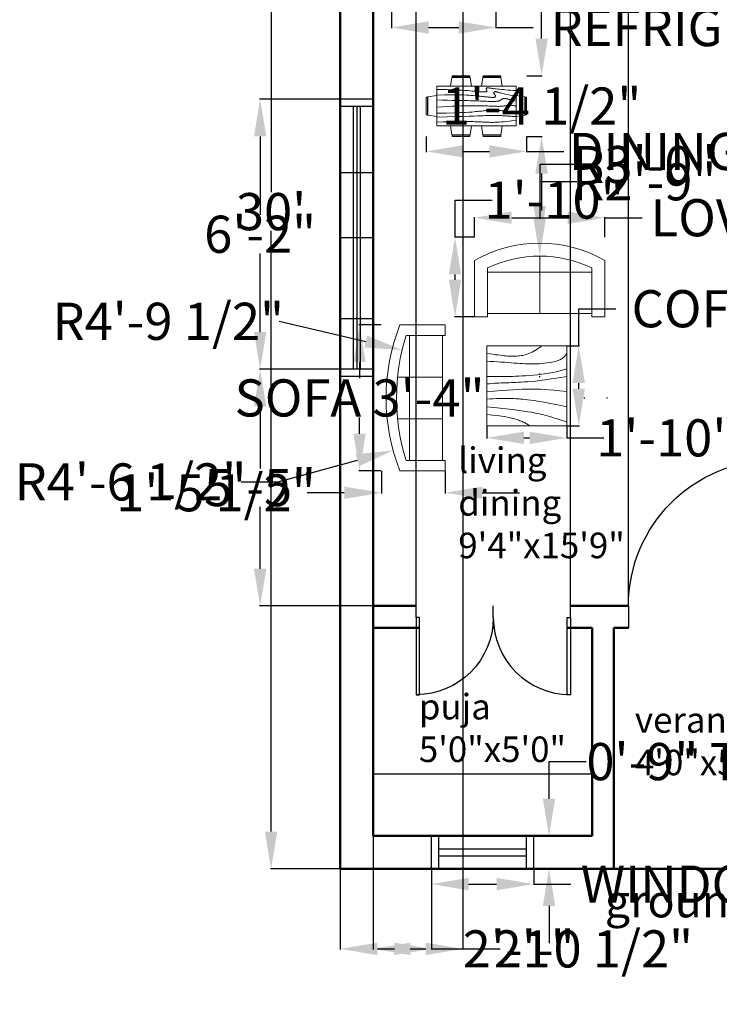
# Model space of a CAD drawing. Units: inches. Extents: x 19 to 1371, y 7 to 588.
# Tile 1 of 5: x 879 to 1070, y 103 to 372. Entities that reach past the tile are written whole.
import ezdxf

# ---------------------------------------------------------------- set-up
doc = ezdxf.new("R2010")
doc.units = ezdxf.units.IN
doc.header["$MEASUREMENT"] = 0
for name, color, linetype, lineweight in [('A-ANNO-DIMS', 2, 'Continuous', 18), ('A-ANNO-TEXT', 7, 'Continuous', 18), ('A-AREA-IDEN', 7, 'Continuous', 18), ('A-DOOR', 3, 'Continuous', 25), ('A-FLOR-CABN', 8, 'Continuous', 25), ('A-FURN', 8, 'Continuous', 18), ('A-GLAZ', 4, 'Continuous', 25), ('A-WALL', 7, 'Continuous', 50)]:
    doc.layers.add(name, color=color, linetype=linetype, lineweight=lineweight)
doc.styles.get("Standard").update_dxf_attribs({"font": 'arial.ttf'})
doc.dimstyles.get("Standard").update_dxf_attribs({"dimtxt": 10.18, "dimasz": 10.18, "dimexe": 0.18, "dimexo": 0.0625, "dimgap": 0.09, "dimtad": 0, "dimtih": 1, "dimtoh": 1, "dimdec": 0, "dimzin": 0, "dimdsep": 46, "dimlunit": 3, "dimtxsty": 'Standard', "dimcen": 0.09, "dimadec": 0, "dimazin": 0, "dimtfac": 1, "dimtdec": 0, "dimtofl": 0, "dimtmove": 0, "dimatfit": 3, "dimfxl": 1, "dimtolj": 1, "dimtzin": 0, "dimarcsym": 0})

# ---------------------------------------------------------------- blocks, each defined once
blk = doc.blocks.new('*U2')
for p, q in [((0, 0), (0, -6)), ((40, 0), (40, -6))]:
    blk.add_line(p, q)
blk.add_lwpolyline([(0, 0), (0, 40), (1.75, 40), (1.75, 0)], close=True)
blk.add_arc((0, 0), 40, 0, 90)
blk = doc.blocks.new('Dining Set - 36 x 72 in.')
for p, q in [((-22, 27.5), (-22.1562, 26.50042)), ((-22, 27.5), (-6, 27.5)), ((-5.8437, 26.49966), (-6, 27.5)), ((6, 27.5), (5.8438, 26.50042)), ((6, 27.5), (22, 27.5)), ((22.1563, 26.49966), (22, 27.5)), ((36, 18), (-36, 18)), ((-36, 18), (-36, -18)), ((-22.2343, 26.00059), (-23.4847, 17.99762)), ((-22.2304, 26), (-5.7608, 26)), ((-5.8416, 26.5), (-22.1534, 26.5)), ((-4.5152, 17.99762), (-5.7655, 25.99926)), ((5.7657, 26.00059), (4.5153, 17.99762)), ((5.7696, 26), (22.2392, 26)), ((22.1584, 26.5), (5.8466, 26.5)), ((23.4848, 17.99762), (22.2345, 25.99926)), ((36, -18), (36, 18)), ((-44.0006, 8.23428), (-35.9976, 9.48474)), ((44.0006, 8.23428), (35.9976, 9.48474)), ((-45.5, 8), (-44.5004, 8.15617)), ((-45.5, 8), (-45.5, -8)), ((-44.5, -8.15843), (-44.5, 8.15338)), ((-44, 8.23041), (-44, -8.23915)), ((44, 8.23041), (44, -8.23915)), ((44.5, -8.15843), (44.5, 8.15338)), ((45.5, 8), (44.5005, 8.15617)), ((45.5, 8), (45.5, -8)), ((-44.4997, -8.15631), (-45.5, -8)), ((-35.9976, -9.48476), (-43.9993, -8.2345)), ((35.9976, -9.48476), (43.9993, -8.2345)), ((44.4997, -8.15631), (45.5, -8)), ((-36, -18), (36, -18)), ((-22.2343, -26.0006), (-23.4847, -17.99762)), ((-22.2304, -26), (-5.7608, -26)), ((-22, -27.5), (-22.1562, -26.50044)), ((-5.8416, -26.5), (-22.1534, -26.5)), ((-5.8437, -26.49967), (-6, -27.5)), ((-4.5152, -17.99762), (-5.7655, -25.99928)), ((5.7657, -26.0006), (4.5153, -17.99762)), ((5.7696, -26), (22.2392, -26)), ((6, -27.5), (5.8438, -26.50044)), ((22.1584, -26.5), (5.8466, -26.5)), ((22.1563, -26.49967), (22, -27.5)), ((23.4848, -17.99762), (22.2345, -25.99928)), ((-22, -27.5), (-6, -27.5)), ((6, -27.5), (22, -27.5))]:
    blk.add_line(p, q)
for points in [[(-36, 15), (-31.1772, 14.97754), (-26.8079, 14.91406), (-22.8538, 14.81543), (-19.276, 14.6875), (-16.0362, 14.53613), (-13.0957, 14.36718), (-10.4159, 14.18652), (-7.9583, 14), (-5.6904, 13.81315), (-3.6035, 13.63021), (-1.6954, 13.45508), (0.0365, 13.29166), (1.5945, 13.14388), (2.9811, 13.01562), (4.1988, 12.9108), (5.25, 12.83333), (6.1393, 12.78613), (6.8802, 12.76823), (7.4883, 12.77767), (7.9792, 12.8125), (8.3685, 12.87077), (8.6719, 12.95052), (8.9049, 13.0498), (9.0833, 13.16666), (9.2205, 13.29899), (9.3216, 13.44401), (9.3895, 13.59879), (9.4271, 13.76041), (9.4373, 13.92594), (9.4232, 14.09245), (9.3875, 14.257), (9.3333, 14.41666), (9.2638, 14.56917), (9.1836, 14.71484), (9.0975, 14.85465), (9.0104, 14.98958), (8.9272, 15.1206), (8.8529, 15.2487), (8.7922, 15.37483), (8.75, 15.5), (8.7305, 15.62467), (8.7344, 15.74739), (8.7617, 15.86621), (8.8125, 15.97916), (8.8867, 16.08431), (8.9844, 16.17968), (9.1055, 16.26334), (9.25, 16.33333), (9.4189, 16.38802), (9.6172, 16.42708), (9.8506, 16.45052), (10.125, 16.45833), (10.4463, 16.45052), (10.8203, 16.42708), (11.2529, 16.38802), (11.75, 16.33333), (12.3184, 16.26318), (12.9694, 16.17838), (13.7151, 16.07991), (14.5677, 15.96875), (15.5395, 15.84586), (16.6426, 15.71224), (17.8893, 15.56884), (19.2917, 15.41666), (20.859, 15.25667), (22.5879, 15.08984), (24.4721, 14.91715), (26.5052, 14.73958), (28.6809, 14.5581), (30.9929, 14.3737), (33.4347, 14.18733), (36, 14)], [(-36, 10), (-28.9766, 10.14274), (-23.1725, 10.20442), (-18.4241, 10.19775), (-14.5677, 10.13541), (-11.4399, 10.03011), (-8.877, 9.89453), (-6.7154, 9.74137), (-4.7917, 9.58333), (-2.9698, 9.43082), (-1.2246, 9.28515), (0.4415, 9.14534), (2.026, 9.01041), (3.5266, 8.87939), (4.9408, 8.7513), (6.266, 8.62516), (7.5, 8.5), (8.6411, 8.37549), (9.6914, 8.2539), (10.6538, 8.13818), (11.5312, 8.03125), (12.3267, 7.93603), (13.043, 7.85547), (13.6831, 7.79248), (14.25, 7.75), (14.7471, 7.7303), (15.1797, 7.73307), (15.5537, 7.75732), (15.875, 7.80208), (16.1494, 7.86637), (16.3828, 7.94922), (16.5811, 8.04964), (16.75, 8.16666), (16.8944, 8.29915), (17.0143, 8.44531), (17.1089, 8.60319), (17.1771, 8.77083), (17.218, 8.94629), (17.2305, 9.1276), (17.2137, 9.31282), (17.1667, 9.5), (17.0895, 9.6875), (16.987, 9.875), (16.8649, 10.0625), (16.7292, 10.25), (16.5856, 10.4375), (16.4401, 10.625), (16.2985, 10.8125), (16.1667, 11), (16.05, 11.18733), (15.9518, 11.3737), (15.8752, 11.5581), (15.8229, 11.73958), (15.798, 11.91715), (15.8034, 12.08984), (15.842, 12.25667), (15.9167, 12.41666), (16.0295, 12.56836), (16.1784, 12.70833), (16.3605, 12.83268), (16.5729, 12.9375), (16.8127, 13.01888), (17.0768, 13.07291), (17.3625, 13.0957), (17.6667, 13.08333), (17.9894, 13.03312), (18.3418, 12.94726), (18.7382, 12.82918), (19.1927, 12.68229), (19.7195, 12.51001), (20.3327, 12.31575), (21.0465, 12.10294), (21.875, 11.875), (22.8357, 11.63354), (23.959, 11.37304), (25.2786, 11.08618), (26.8282, 10.76562), (28.6414, 10.40405), (30.752, 9.99414), (33.1936, 9.52856), (36, 9)], [(-36, 5.5), (-30.7157, 5.3348), (-26.069, 5.20963), (-21.9946, 5.11767), (-18.4271, 5.05208), (-15.3009, 5.00602), (-12.5508, 4.97265), (-10.1112, 4.94515), (-7.9167, 4.91666), (-5.909, 4.88167), (-4.0586, 4.83984), (-2.3429, 4.79215), (-0.7396, 4.73958), (0.7739, 4.6831), (2.22, 4.6237), (3.6213, 4.56233), (5, 4.5), (6.373, 4.43782), (7.7344, 4.3776), (9.0723, 4.32129), (10.375, 4.27083), (11.6309, 4.22819), (12.8281, 4.19531), (13.9551, 4.17415), (15, 4.16666), (15.954, 4.17448), (16.819, 4.19791), (17.6001, 4.23698), (18.3021, 4.29166), (18.9299, 4.36198), (19.4883, 4.44791), (19.9823, 4.54948), (20.4167, 4.66666), (20.7969, 4.79899), (21.1302, 4.94401), (21.4245, 5.09879), (21.6875, 5.26041), (21.9271, 5.42594), (22.1511, 5.59245), (22.3672, 5.757), (22.5834, 5.91666), (22.8065, 6.06868), (23.0404, 6.21093), (23.2879, 6.34147), (23.5521, 6.45833), (23.8358, 6.55957), (24.142, 6.64323), (24.4735, 6.70735), (24.8334, 6.75), (25.2235, 6.76969), (25.642, 6.76692), (26.0858, 6.74267), (26.5521, 6.69791), (27.0379, 6.63362), (27.5404, 6.55078), (28.0565, 6.45036), (28.5834, 6.33333), (29.1242, 6.19987), (29.7071, 6.04687), (30.3661, 5.87044), (31.1354, 5.66666), (32.0493, 5.43164), (33.142, 5.16146), (34.4475, 4.85221), (36, 4.5)], [(-36, -1), (-30.7915, -0.6591), (-26.0195, -0.38216), (-21.6519, -0.16284), (-17.6563, 0.00521), (-14.0005, 0.12833), (-10.6523, 0.21289), (-7.5796, 0.26522), (-4.75, 0.29166), (-2.134, 0.29793), (0.2878, 0.28711), (2.5317, 0.26163), (4.6146, 0.22396), (6.5529, 0.17651), (8.3633, 0.12174), (10.0623, 0.06209), (11.6667, 0), (13.1899, -0.06201), (14.6341, -0.1211), (15.9982, -0.17432), (17.2813, -0.21875), (18.4823, -0.25147), (19.6003, -0.26953), (20.6343, -0.27002), (21.5834, -0.25), (22.4481, -0.20768), (23.2357, -0.14584), (23.9549, -0.06836), (24.6146, 0.02083), (25.2235, 0.11784), (25.7904, 0.21875), (26.3241, 0.31966), (26.8334, 0.41666), (27.3265, 0.50618), (27.8099, 0.58593), (28.2894, 0.65397), (28.7709, 0.70833), (29.2601, 0.74707), (29.763, 0.76823), (30.2855, 0.76985), (30.8334, 0.75), (31.4088, 0.70784), (31.9994, 0.64713), (32.589, 0.57275), (33.1615, 0.48958), (33.7008, 0.4025), (34.1908, 0.3164), (34.6153, 0.23616), (34.9584, 0.16666), (35.2099, 0.11165), (35.3848, 0.07031), (35.504, 0.04069), (35.5886, 0.02083), (35.6594, 0.00879), (35.7377, 0.0026), (35.8442, 0.00032), (36, 0)], [(-36, -6.5), (-27.1843, -6.31267), (-20.084, -6.1263), (-14.469, -5.9419), (-10.1094, -5.76042), (-6.7752, -5.58285), (-4.2363, -5.41016), (-2.2629, -5.24333), (-0.625, -5.08334), (0.8708, -4.93099), (2.2715, -4.78646), (3.5872, -4.64974), (4.8281, -4.52084), (6.0046, -4.39974), (7.127, -4.28646), (8.2053, -4.18099), (9.25, -4.08334), (10.2705, -3.99382), (11.2734, -3.91407), (12.2647, -3.84603), (13.25, -3.79167), (14.2354, -3.75293), (15.2266, -3.73177), (16.2295, -3.73015), (17.25, -3.75), (18.2912, -3.79248), (19.3451, -3.85547), (20.4009, -3.93604), (21.4479, -4.03125), (22.4754, -4.13819), (23.4727, -4.25391), (24.4289, -4.37549), (25.3334, -4.5), (26.1785, -4.62492), (26.9694, -4.74935), (27.7145, -4.87281), (28.4219, -4.99479), (29.1, -5.11483), (29.7572, -5.23242), (30.4016, -5.34709), (31.0417, -5.45834), (31.6837, -5.56437), (32.3262, -5.65821), (32.9658, -5.73153), (33.599, -5.77604), (34.2224, -5.78345), (34.8327, -5.74545), (35.4264, -5.65373), (36, -5.5)], [(-36, -10), (-26.4022, -9.81299), (-18.4675, -9.62891), (-11.9839, -9.45069), (-6.7396, -9.28125), (-2.5226, -9.12354), (0.8789, -8.98047), (3.6769, -8.85498), (6.0833, -8.75), (8.2767, -8.66765), (10.3021, -8.60677), (12.1712, -8.56543), (13.8958, -8.54167), (15.4876, -8.53353), (16.9583, -8.53907), (18.3197, -8.55632), (19.5834, -8.58334), (20.7616, -8.61841), (21.8685, -8.66081), (22.9188, -8.71004), (23.9271, -8.76563), (24.9081, -8.82707), (25.8763, -8.89388), (26.8465, -8.96558), (27.8334, -9.04167), (28.8474, -9.12118), (29.8828, -9.20117), (30.93, -9.27824), (31.9792, -9.34896), (33.0205, -9.40991), (34.0443, -9.45768), (35.0407, -9.48885), (36, -9.5)], [(-36, -14.5), (-30.0881, -14.33513), (-25.0332, -14.21224), (-20.7312, -14.12647), (-17.0781, -14.07292), (-13.97, -14.04671), (-11.3027, -14.04297), (-8.9724, -14.05681), (-6.875, -14.08334), (-4.9224, -14.11833), (-3.0905, -14.16016), (-1.3709, -14.20785), (0.2448, -14.26042), (1.7647, -14.3169), (3.1973, -14.3763), (4.5507, -14.43767), (5.8333, -14.5), (7.0554, -14.5621), (8.235, -14.62175), (9.3922, -14.67652), (10.5469, -14.72396), (11.7192, -14.76164), (12.929, -14.78711), (14.1965, -14.79794), (15.5417, -14.79167), (16.9933, -14.76424), (18.6152, -14.70508), (20.4804, -14.60197), (22.6615, -14.44271), (25.2312, -14.21509), (28.2624, -13.9069), (31.8277, -13.50594), (36, -13)]]:
    blk.add_lwpolyline(points)
blk = doc.blocks.new('Sofa - Roundback 7 ft.')
for p, q in [((-12.00002, -32.4421), (-12.00003, -6.5971)), ((11.99997, -32.4421), (11.99998, -6.5971)), ((-36.000027, -34), (-36.000027, -11.4696)), ((-35.999844, -13.3819), (35.9998, -13.3819)), ((35.99998, -34), (35.99998, -11.4696)), ((-36.000027, -32.4421), (35.99998, -32.4421))]:
    blk.add_line(p, q)
for points in [[(-36.000027, -34), (-42.000027, -34), (-42.000027, -8)], [(41.99998, -8), (41.99998, -34), (35.99998, -34)]]:
    blk.add_lwpolyline(points)
for centre, radius, start, end in [((0, -114.25), 114.25, 68.43141, 111.5686), ((-0.00001, -127.1968), 121.1968, 72.72033, 107.2797)]:
    blk.add_arc(centre, radius, start, end)
blk = doc.blocks.new('Sofa - Roundback Loveseat 5 ft.')
for p, q in [((0, -32.44198), (0, -5.99998)), ((-24, -33.99998), (-24, -11.46958)), ((-23.9998, -13.38178), (23.99986, -13.38178)), ((24.00004, -33.99998), (24.00004, -11.46958)), ((-24, -32.44198), (24.00004, -32.44198))]:
    blk.add_line(p, q)
for points in [[(-24, -33.99998), (-30, -33.99998), (-30, -7.99998)], [(30.00004, -7.99998), (30.00004, -33.99998), (24.00004, -33.99998)]]:
    blk.add_lwpolyline(points)
for centre, radius, start, end in [((0, -60.24998), 60.24998, 60.13715, 119.8628), ((0, -61.38438), 55.38444, 64.32083, 115.6792)]:
    blk.add_arc(centre, radius, start, end)
blk = doc.blocks.new('Table - Square Woodgrain 42 x 42 in.')
blk.add_line((0, -42), (42, -42))
for points in [[(0, -4), (1.704, -4.2172), (3.2358, -4.4188), (4.615, -4.604), (5.8615, -4.7721), (6.9951, -4.9224), (8.0357, -5.0541), (9.0031, -5.1667), (9.9171, -5.2594), (10.7951, -5.3316), (11.6445, -5.3836), (12.4702, -5.4157), (13.277, -5.4283), (14.0698, -5.4217), (14.8535, -5.3964), (15.6331, -5.3526), (16.4133, -5.2908), (17.1986, -5.2103), (17.9913, -5.1062), (18.793, -4.9727), (19.6056, -4.8038), (20.4307, -4.5937), (21.2701, -4.3365), (22.1256, -4.0262), (22.9989, -3.6571), (23.888, -3.2272), (24.7756, -2.7516), (25.6408, -2.2491), (26.4624, -1.7387), (27.2195, -1.2395), (27.891, -0.7703), (28.456, -0.3501), (28.8934, 0.002)], [(0, -42), (0, 0), (42, 0), (42, -42)], [(0, -8), (1.8203, -8.1001), (3.6741, -8.2149), (5.5411, -8.3408), (7.4011, -8.4741), (9.2339, -8.6112), (11.0193, -8.7484), (12.7371, -8.8821), (14.3671, -9.0086), (15.8954, -9.1246), (17.3337, -9.2278), (18.6997, -9.3159), (20.0116, -9.387), (21.2871, -9.4389), (22.5442, -9.4696), (23.8008, -9.477), (25.0749, -9.459), (26.3791, -9.4137), (27.7049, -9.3403), (29.0383, -9.2382), (30.3655, -9.1068), (31.6728, -8.9455), (32.9461, -8.7535), (34.1717, -8.5304), (35.3358, -8.2756), (36.4268, -7.9863), (37.443, -7.6521), (38.3849, -7.2603), (39.253, -6.7986), (40.048, -6.2542), (40.7705, -5.6147), (41.421, -4.8674), (42, -4)], [(42, -12), (39.1784, -12.8621), (36.4519, -13.5654), (33.8246, -14.1294), (31.3004, -14.5731), (28.8832, -14.9161), (26.577, -15.1775), (24.3858, -15.3768), (22.3136, -15.5332), (20.3622, -15.6632), (18.5254, -15.7718), (16.7947, -15.8612), (15.1618, -15.9338), (13.6183, -15.9916), (12.1558, -16.0369), (10.7659, -16.0718), (9.4403, -16.0987), (8.1703, -16.1191), (6.9461, -16.1325), (5.7577, -16.1377), (4.595, -16.1335), (3.4479, -16.1188), (2.3064, -16.0924), (1.1604, -16.0532), (0, -16)], [(42, -16), (37.6529, -16.7365), (33.8802, -17.329), (30.6179, -17.7961), (27.8015, -18.1561), (25.3668, -18.4275), (23.2497, -18.6288), (21.3859, -18.7785), (19.7111, -18.8949), (18.1693, -18.9939), (16.7375, -19.0795), (15.401, -19.1534), (14.1449, -19.217), (12.9544, -19.2717), (11.8148, -19.3191), (10.7113, -19.3606), (9.6291, -19.3976), (8.5534, -19.4323), (7.47, -19.4689), (6.3643, -19.5122), (5.222, -19.5672), (4.0288, -19.6386), (2.7703, -19.7313), (1.4321, -19.8501), (0, -20)], [(0, -24), (3.9243, -23.6805), (7.4766, -23.4138), (10.6891, -23.1954), (13.5943, -23.0205), (16.2247, -22.8847), (18.6125, -22.7832), (20.7903, -22.7116), (22.7903, -22.6651), (24.6563, -22.642), (26.4764, -22.6507), (28.35, -22.7024), (30.3766, -22.8084), (32.6555, -22.98), (35.2861, -23.2283), (38.3678, -23.5645), (42, -24)], [(42, -32), (37.392, -31.017), (33.4585, -30.2231), (30.1291, -29.5949), (27.3334, -29.109), (25.0009, -28.742), (23.0612, -28.4707), (21.4439, -28.2716), (20.0786, -28.1215), (18.8998, -28.0002), (17.8609, -27.9014), (16.9206, -27.8219), (16.0371, -27.7588), (15.1691, -27.709), (14.2748, -27.6693), (13.3128, -27.6368), (12.2415, -27.6083), (11.0295, -27.5824), (9.6867, -27.5643), (8.233, -27.5608), (6.6884, -27.5787), (5.0728, -27.6248), (3.4062, -27.7058), (1.7086, -27.8286), (0, -28)], [(0, -32), (5.4026, -32.5358), (9.9494, -33.019), (13.7424, -33.4553), (16.8834, -33.8505), (19.4743, -34.2106), (21.6171, -34.5413), (23.4136, -34.8486), (24.9657, -35.1382), (26.3614, -35.4156), (27.6332, -35.6841), (28.7995, -35.9467), (29.8788, -36.2064), (30.8897, -36.4661), (31.8507, -36.7288), (32.7802, -36.9973), (33.6968, -37.2747), (34.6175, -37.5635), (35.5531, -37.8651), (36.5128, -38.1805), (37.506, -38.5108), (38.5421, -38.8568), (39.6302, -39.2197), (40.7797, -39.6004), (42, -40)], [(0, -36), (3.0098, -36.2857), (5.5354, -36.5643), (7.6368, -36.8359), (9.374, -37.1009), (10.807, -37.3597), (11.9957, -37.6126), (13.0002, -37.8599), (13.8804, -38.102), (14.6874, -38.3393), (15.4365, -38.5729), (16.1338, -38.8041), (16.7858, -39.0341), (17.3987, -39.264), (17.9787, -39.4952), (18.5322, -39.7288), (19.0655, -39.9662), (19.5832, -40.2081), (20.0842, -40.4544), (20.5657, -40.7046), (21.0249, -40.9581), (21.459, -41.2144), (21.8653, -41.4731), (22.2409, -41.7335), (22.5831, -41.9951)]]:
    blk.add_lwpolyline(points)
blk = doc.blocks.new('*D14')
at = {"layer": 'A-ANNO-DIMS', "color": 0, "lineweight": -2, "transparency": 16777216}
for p, q in [((966.38, 499.95), (947.31, 499.95)), ((947.49, 489.77), (947.49, 325.21)), ((947.49, 150.07), (947.49, 314.63)), ((966.38, 139.89), (947.31, 139.89))]:
    blk.add_line(p, q, dxfattribs=at)
at = {"layer": 'A-ANNO-DIMS', "color": 0, "transparency": 16777216}
for points in [[(945.79, 489.77), (949.18, 489.77), (947.49, 499.95)], [(945.79, 150.07), (949.18, 150.07), (947.49, 139.89)]]:
    blk.add_solid(points, dxfattribs=at)
at = {"layer": 'Defpoints', "color": 0, "transparency": 16777216}
for p in [(966.44, 499.95), (947.49, 139.89), (966.44, 139.89)]:
    blk.add_point(p, dxfattribs=at)
at = {"layer": 'A-ANNO-DIMS', "color": 0, "transparency": 16777216, "insert": (947.49, 319.92), "char_height": 10.18, "attachment_point": 5}
blk.add_mtext("\\A1;30'", dxfattribs=at)
blk = doc.blocks.new('WIN-24')
for p, q in [((0, 0), (0, 9)), ((2, 0), (2, 9)), ((26, 0), (26, 9)), ((28, 0), (28, 9)), ((2, 5.5), (26, 5.5)), ((2, 3.5), (26, 3.5))]:
    blk.add_line(p, q)
blk = doc.blocks.new('*D26')
at = {"layer": 'A-ANNO-DIMS', "color": 0, "lineweight": -2, "transparency": 16777216}
for p, q in [((991.44, 139.83), (991.44, 135.51)), ((1019.44, 139.83), (1019.44, 135.51)), ((1001.62, 135.69), (1009.26, 135.69)), ((1019.44, 135.69), (1029.62, 135.69))]:
    blk.add_line(p, q, dxfattribs=at)
at = {"layer": 'A-ANNO-DIMS', "color": 0, "transparency": 16777216}
for points in [[(1001.62, 137.39), (1001.62, 133.99), (991.44, 135.69)], [(1009.26, 137.39), (1009.26, 133.99), (1019.44, 135.69)]]:
    blk.add_solid(points, dxfattribs=at)
at = {"layer": 'Defpoints', "color": 0, "transparency": 16777216}
for p in [(991.44, 139.89), (1019.44, 139.89), (1019.44, 135.69)]:
    blk.add_point(p, dxfattribs=at)
at = {"layer": 'A-ANNO-DIMS', "color": 0, "transparency": 16777216, "insert": (1094.12, 135.69), "char_height": 10.18, "attachment_point": 5}
blk.add_mtext('\\A1;WINDOW 2\'-4" TYP.', dxfattribs=at)
blk = doc.blocks.new('*D27')
at = {"layer": 'A-ANNO-DIMS', "color": 0, "lineweight": -2, "transparency": 16777216}
for p, q in [((1023.64, 159.07), (1023.64, 169.25)), ((1023.64, 169.25), (1033.82, 169.25)), ((1019.5, 148.89), (1023.82, 148.89)), ((1019.5, 139.89), (1023.82, 139.89)), ((1023.64, 129.71), (1023.64, 119.53))]:
    blk.add_line(p, q, dxfattribs=at)
at = {"layer": 'A-ANNO-DIMS', "color": 0, "transparency": 16777216}
for points in [[(1021.95, 159.07), (1025.34, 159.07), (1023.64, 148.89)], [(1021.95, 129.71), (1025.34, 129.71), (1023.64, 139.89)]]:
    blk.add_solid(points, dxfattribs=at)
at = {"layer": 'Defpoints', "color": 0, "transparency": 16777216}
for p in [(1019.44, 148.89), (1023.64, 148.89), (1019.44, 139.89)]:
    blk.add_point(p, dxfattribs=at)
at = {"layer": 'A-ANNO-DIMS', "color": 0, "transparency": 16777216, "insert": (1064.94, 169.25), "char_height": 10.18, "attachment_point": 5}
blk.add_mtext('\\A1;0\'-9" TYP.', dxfattribs=at)
blk = doc.blocks.new('*D36')
at = {"layer": 'A-ANNO-DIMS', "color": 0, "lineweight": -2, "transparency": 16777216}
for p, q in [((980.44, 374.59), (980.44, 370.17)), ((1009.08, 374.59), (1009.08, 370.17)), ((990.62, 370.35), (998.9, 370.35)), ((1009.08, 370.35), (1019.26, 370.35))]:
    blk.add_line(p, q, dxfattribs=at)
at = {"layer": 'A-ANNO-DIMS', "color": 0, "transparency": 16777216}
for points in [[(990.62, 372.05), (990.62, 368.66), (980.44, 370.35)], [(998.9, 372.05), (998.9, 368.66), (1009.08, 370.35)]]:
    blk.add_solid(points, dxfattribs=at)
at = {"layer": 'Defpoints', "color": 0, "transparency": 16777216}
for p in [(980.44, 374.65), (1009.08, 374.65), (1009.08, 370.35)]:
    blk.add_point(p, dxfattribs=at)
at = {"layer": 'A-ANNO-DIMS', "color": 0, "transparency": 16777216, "insert": (1102.94, 370.35), "char_height": 10.18, "attachment_point": 5}
blk.add_mtext('\\A1;REFRIGERATOR 2\'-4 1/2"', dxfattribs=at)
blk = doc.blocks.new('*D38')
at = {"layer": 'A-ANNO-DIMS', "color": 0, "lineweight": -2, "transparency": 16777216}
for p, q in [((990.01, 340.47), (990.01, 336.23)), ((1017.49, 340.47), (1017.49, 336.23)), ((1000.19, 336.41), (1007.31, 336.41)), ((1017.49, 336.41), (1027.67, 336.41))]:
    blk.add_line(p, q, dxfattribs=at)
at = {"layer": 'A-ANNO-DIMS', "color": 0, "transparency": 16777216}
for points in [[(1000.19, 338.11), (1000.19, 334.72), (990.01, 336.41)], [(1007.31, 338.11), (1007.31, 334.72), (1017.49, 336.41)]]:
    blk.add_solid(points, dxfattribs=at)
at = {"layer": 'Defpoints', "color": 0, "transparency": 16777216}
for p in [(990.01, 340.54), (1017.49, 340.54), (1017.49, 336.41)]:
    blk.add_point(p, dxfattribs=at)
at = {"layer": 'A-ANNO-DIMS', "color": 0, "transparency": 16777216, "insert": (1095.56, 336.41), "char_height": 10.18, "attachment_point": 5}
blk.add_mtext('\\A1;DINING SET 2\'-3 1/2"', dxfattribs=at)
blk = doc.blocks.new('*D39')
at = {"layer": 'A-ANNO-DIMS', "color": 0, "lineweight": -2, "transparency": 16777216}
for p, q in [((1021.61, 367.32), (1021.61, 377.5)), ((1017.55, 357.14), (1021.79, 357.14)), ((1017.55, 340.54), (1021.79, 340.54)), ((1021.61, 330.36), (1021.61, 320.18))]:
    blk.add_line(p, q, dxfattribs=at)
at = {"layer": 'A-ANNO-DIMS', "color": 0, "transparency": 16777216}
for points in [[(1019.91, 367.32), (1023.31, 367.32), (1021.61, 357.14)], [(1019.91, 330.36), (1023.31, 330.36), (1021.61, 340.54)]]:
    blk.add_solid(points, dxfattribs=at)
at = {"layer": 'Defpoints', "color": 0, "transparency": 16777216}
for p in [(1017.49, 357.14), (1021.61, 357.14), (1017.49, 340.54)]:
    blk.add_point(p, dxfattribs=at)
at = {"layer": 'A-ANNO-DIMS', "color": 0, "transparency": 16777216, "insert": (1021.61, 348.84), "char_height": 10.18, "attachment_point": 5}
blk.add_mtext('\\A1;1\'-4 1/2"', dxfattribs=at)
blk = doc.blocks.new('*D40')
at = {"layer": 'A-ANNO-DIMS', "color": 0, "lineweight": -2, "transparency": 16777216}
for p, q in [((977.67, 288.87), (971.55, 288.87)), ((971.73, 278.69), (971.73, 274.25)), ((971.73, 259.08), (971.73, 263.52)), ((977.67, 248.9), (971.55, 248.9))]:
    blk.add_line(p, q, dxfattribs=at)
at = {"layer": 'A-ANNO-DIMS', "color": 0, "transparency": 16777216}
for points in [[(970.04, 278.69), (973.43, 278.69), (971.73, 288.87)], [(970.04, 259.08), (973.43, 259.08), (971.73, 248.9)]]:
    blk.add_solid(points, dxfattribs=at)
at = {"layer": 'Defpoints', "color": 0, "transparency": 16777216}
for p in [(971.73, 288.87), (977.73, 288.87), (977.73, 248.9)]:
    blk.add_point(p, dxfattribs=at)
at = {"layer": 'A-ANNO-DIMS', "color": 0, "transparency": 16777216, "insert": (971.73, 268.88), "char_height": 10.18, "attachment_point": 5}
blk.add_mtext('\\A1;SOFA 3\'-4"', dxfattribs=at)
blk = doc.blocks.new('*D41')
at = {"layer": 'A-ANNO-DIMS', "color": 0, "lineweight": -2, "transparency": 16777216}
for p, q in [((977.73, 248.83), (977.73, 242.72)), ((995.18, 248.83), (995.18, 242.72)), ((967.55, 242.9), (957.37, 242.9)), ((1005.36, 242.9), (1015.54, 242.9))]:
    blk.add_line(p, q, dxfattribs=at)
at = {"layer": 'A-ANNO-DIMS', "color": 0, "transparency": 16777216}
for points in [[(967.55, 244.59), (967.55, 241.2), (977.73, 242.9)], [(1005.36, 244.59), (1005.36, 241.2), (995.18, 242.9)]]:
    blk.add_solid(points, dxfattribs=at)
at = {"layer": 'Defpoints', "color": 0, "transparency": 16777216}
for p in [(977.73, 248.9), (995.18, 248.9), (977.73, 242.9)]:
    blk.add_point(p, dxfattribs=at)
at = {"layer": 'A-ANNO-DIMS', "color": 0, "transparency": 16777216, "insert": (932.37, 242.9), "char_height": 10.18, "attachment_point": 5}
blk.add_mtext('\\A1;1\'-5 1/2"', dxfattribs=at)
blk = doc.blocks.new('*D42')
at = {"layer": 'A-ANNO-DIMS', "color": 0, "lineweight": -2, "transparency": 16777216}
for p, q in [((1003.24, 312.95), (1003.24, 318.42)), ((1038.94, 312.95), (1038.94, 318.42)), ((1013.42, 318.24), (1028.76, 318.24)), ((1038.94, 318.24), (1049.12, 318.24))]:
    blk.add_line(p, q, dxfattribs=at)
at = {"layer": 'A-ANNO-DIMS', "color": 0, "transparency": 16777216}
for points in [[(1013.42, 319.94), (1013.42, 316.55), (1003.24, 318.24)], [(1028.76, 319.94), (1028.76, 316.55), (1038.94, 318.24)]]:
    blk.add_solid(points, dxfattribs=at)
at = {"layer": 'Defpoints', "color": 0, "transparency": 16777216}
for p in [(1038.94, 318.24), (1003.24, 312.89), (1038.94, 312.89)]:
    blk.add_point(p, dxfattribs=at)
at = {"layer": 'A-ANNO-DIMS', "color": 0, "transparency": 16777216, "insert": (1117.85, 318.24), "char_height": 10.18, "attachment_point": 5}
blk.add_mtext('\\A1;LOVESEAT 2\'-11 1/2"', dxfattribs=at)
blk = doc.blocks.new('*D43')
at = {"layer": 'A-ANNO-DIMS', "color": 0, "lineweight": -2, "transparency": 16777216}
for p, q in [((997.88, 312.89), (997.88, 323.07)), ((997.88, 323.07), (1008.06, 323.07)), ((1003.17, 312.89), (997.7, 312.89)), ((997.88, 301.25), (997.88, 302.71)), ((1003.17, 291.07), (997.7, 291.07))]:
    blk.add_line(p, q, dxfattribs=at)
at = {"layer": 'A-ANNO-DIMS', "color": 0, "transparency": 16777216}
for points in [[(996.18, 302.71), (999.58, 302.71), (997.88, 312.89)], [(996.18, 301.25), (999.58, 301.25), (997.88, 291.07)]]:
    blk.add_solid(points, dxfattribs=at)
at = {"layer": 'Defpoints', "color": 0, "transparency": 16777216}
for p in [(997.88, 312.89), (1003.24, 312.89), (1003.24, 291.07)]:
    blk.add_point(p, dxfattribs=at)
at = {"layer": 'A-ANNO-DIMS', "color": 0, "transparency": 16777216, "insert": (1025.16, 323.07), "char_height": 10.18, "attachment_point": 5}
blk.add_mtext('\\A1;1\'-10"', dxfattribs=at)
blk = doc.blocks.new('*D44')
at = {"layer": 'A-ANNO-DIMS', "color": 0, "lineweight": -2, "transparency": 16777216}
for p, q in [((1031.78, 283.13), (1031.78, 293.31)), ((1031.78, 293.31), (1041.96, 293.31)), ((1028.56, 283.13), (1031.96, 283.13)), ((1031.78, 271.4), (1031.78, 272.95)), ((1028.56, 261.22), (1031.96, 261.22))]:
    blk.add_line(p, q, dxfattribs=at)
at = {"layer": 'A-ANNO-DIMS', "color": 0, "transparency": 16777216}
for points in [[(1030.09, 272.95), (1033.48, 272.95), (1031.78, 283.13)], [(1030.09, 271.4), (1033.48, 271.4), (1031.78, 261.22)]]:
    blk.add_solid(points, dxfattribs=at)
at = {"layer": 'Defpoints', "color": 0, "transparency": 16777216}
for p in [(1028.5, 283.13), (1031.78, 283.13), (1028.5, 261.22)]:
    blk.add_point(p, dxfattribs=at)
at = {"layer": 'A-ANNO-DIMS', "color": 0, "transparency": 16777216, "insert": (1114.8, 293.31), "char_height": 10.18, "attachment_point": 5}
blk.add_mtext('\\A1;COFFEE TABLE 1\'-10"', dxfattribs=at)
blk = doc.blocks.new('*D45')
at = {"layer": 'A-ANNO-DIMS', "color": 0, "lineweight": -2, "transparency": 16777216}
for p, q in [((1006.59, 261.16), (1006.59, 257.76)), ((1028.5, 261.16), (1028.5, 257.76)), ((1016.77, 257.94), (1018.32, 257.94)), ((1028.5, 257.94), (1038.68, 257.94))]:
    blk.add_line(p, q, dxfattribs=at)
at = {"layer": 'A-ANNO-DIMS', "color": 0, "transparency": 16777216}
for points in [[(1016.77, 259.63), (1016.77, 256.24), (1006.59, 257.94)], [(1018.32, 259.63), (1018.32, 256.24), (1028.5, 257.94)]]:
    blk.add_solid(points, dxfattribs=at)
at = {"layer": 'Defpoints', "color": 0, "transparency": 16777216}
for p in [(1006.59, 261.22), (1028.5, 261.22), (1028.5, 257.94)]:
    blk.add_point(p, dxfattribs=at)
at = {"layer": 'A-ANNO-DIMS', "color": 0, "transparency": 16777216, "insert": (1055.77, 257.94), "char_height": 10.18, "attachment_point": 5}
blk.add_mtext('\\A1;1\'-10"', dxfattribs=at)
blk = doc.blocks.new('*D46')
at = {"layer": 'A-ANNO-DIMS', "color": 0, "lineweight": -2, "transparency": 16777216}
for p, q in [((1035.21, 572.84), (1025.03, 572.84)), ((1045.39, 211.95), (1045.39, 573.02)), ((1085.39, 211.95), (1085.39, 573.02)), ((1095.57, 572.84), (1105.75, 572.84))]:
    blk.add_line(p, q, dxfattribs=at)
at = {"layer": 'A-ANNO-DIMS', "color": 0, "transparency": 16777216}
for points in [[(1035.21, 574.54), (1035.21, 571.14), (1045.39, 572.84)], [(1095.57, 574.54), (1095.57, 571.14), (1085.39, 572.84)]]:
    blk.add_solid(points, dxfattribs=at)
at = {"layer": 'Defpoints', "color": 0, "transparency": 16777216}
for p in [(1085.39, 572.84), (1045.39, 211.89), (1085.39, 211.89)]:
    blk.add_point(p, dxfattribs=at)
at = {"layer": 'A-ANNO-DIMS', "color": 0, "transparency": 16777216, "insert": (1065.39, 572.84), "char_height": 10.18, "attachment_point": 5}
blk.add_mtext('\\A1;3\'-4"', dxfattribs=at)
blk = doc.blocks.new('*D47')
at = {"layer": 'A-ANNO-DIMS', "color": 0, "lineweight": -2, "transparency": 16777216}
for p, q in [((987.23, 211.95), (987.23, 573.02)), ((997.41, 572.84), (1019.34, 572.84)), ((1029.52, 211.95), (1029.52, 573.02)), ((1029.52, 572.84), (1039.7, 572.84))]:
    blk.add_line(p, q, dxfattribs=at)
at = {"layer": 'A-ANNO-DIMS', "color": 0, "transparency": 16777216}
for points in [[(997.41, 574.54), (997.41, 571.14), (987.23, 572.84)], [(1019.34, 574.54), (1019.34, 571.14), (1029.52, 572.84)]]:
    blk.add_solid(points, dxfattribs=at)
at = {"layer": 'Defpoints', "color": 0, "transparency": 16777216}
for p in [(1029.52, 572.84), (987.23, 211.89), (1029.52, 211.89)]:
    blk.add_point(p, dxfattribs=at)
at = {"layer": 'A-ANNO-DIMS', "color": 0, "transparency": 16777216, "insert": (1065.17, 572.84), "char_height": 10.18, "attachment_point": 5}
blk.add_mtext('\\A1;3\'-6 1/2"', dxfattribs=at)
blk = doc.blocks.new('*D56')
at = {"layer": 'A-ANNO-DIMS', "color": 0, "lineweight": -2, "transparency": 16777216}
for p, q in [((975.44, 406.83), (975.44, 117.76)), ((1000.05, 406.83), (1000.05, 117.76)), ((985.62, 117.94), (989.87, 117.94)), ((1000.05, 117.94), (1010.23, 117.94))]:
    blk.add_line(p, q, dxfattribs=at)
at = {"layer": 'A-ANNO-DIMS', "color": 0, "transparency": 16777216}
for points in [[(985.62, 119.64), (985.62, 116.24), (975.44, 117.94)], [(989.87, 119.64), (989.87, 116.24), (1000.05, 117.94)]]:
    blk.add_solid(points, dxfattribs=at)
at = {"layer": 'Defpoints', "color": 0, "transparency": 16777216}
for p in [(975.44, 406.89), (1000.05, 406.89), (1000.05, 117.94)]:
    blk.add_point(p, dxfattribs=at)
at = {"layer": 'A-ANNO-DIMS', "color": 0, "transparency": 16777216, "insert": (1035.8, 117.94), "char_height": 10.18, "attachment_point": 5}
blk.add_mtext('\\A1;2\'-0 1/2"', dxfattribs=at)
blk = doc.blocks.new('*D59')
at = {"layer": 'A-ANNO-DIMS', "color": 0, "lineweight": -2, "transparency": 16777216}
for p, q in [((966.38, 350.72), (944.31, 350.72)), ((944.49, 340.54), (944.49, 319.01)), ((944.49, 286.9), (944.49, 308.44)), ((966.38, 276.72), (944.31, 276.72))]:
    blk.add_line(p, q, dxfattribs=at)
at = {"layer": 'A-ANNO-DIMS', "color": 0, "transparency": 16777216}
for points in [[(942.8, 340.54), (946.19, 340.54), (944.49, 350.72)], [(942.8, 286.9), (946.19, 286.9), (944.49, 276.72)]]:
    blk.add_solid(points, dxfattribs=at)
at = {"layer": 'Defpoints', "color": 0, "transparency": 16777216}
for p in [(966.44, 350.72), (944.49, 276.72), (966.44, 276.72)]:
    blk.add_point(p, dxfattribs=at)
at = {"layer": 'A-ANNO-DIMS', "color": 0, "transparency": 16777216, "insert": (944.49, 313.72), "char_height": 10.18, "attachment_point": 5}
blk.add_mtext('\\A1;6\'-2"', dxfattribs=at)
blk = doc.blocks.new('*D60')
at = {"layer": 'A-ANNO-DIMS', "color": 0, "lineweight": -2, "transparency": 16777216}
for p, q in [((975.38, 276.72), (944.31, 276.72)), ((944.49, 266.54), (944.49, 249.57)), ((944.49, 222.07), (944.49, 239.04)), ((975.38, 211.89), (944.31, 211.89))]:
    blk.add_line(p, q, dxfattribs=at)
at = {"layer": 'A-ANNO-DIMS', "color": 0, "transparency": 16777216}
for points in [[(942.8, 266.54), (946.19, 266.54), (944.49, 276.72)], [(942.8, 222.07), (946.19, 222.07), (944.49, 211.89)]]:
    blk.add_solid(points, dxfattribs=at)
at = {"layer": 'Defpoints', "color": 0, "transparency": 16777216}
for p in [(944.49, 276.72), (975.44, 276.72), (975.44, 211.89)]:
    blk.add_point(p, dxfattribs=at)
at = {"layer": 'A-ANNO-DIMS', "color": 0, "transparency": 16777216, "insert": (944.49, 244.31), "char_height": 10.18, "attachment_point": 5}
blk.add_mtext('\\A1;5\'-5"', dxfattribs=at)
blk = doc.blocks.new('*D66')
at = {"layer": 'A-ANNO-DIMS', "color": 0, "lineweight": -2, "transparency": 16777216}
for p, q in [((966.44, 139.83), (966.44, 117.76)), ((991.44, 139.83), (991.44, 117.76)), ((976.62, 117.94), (981.26, 117.94)), ((991.44, 117.94), (1001.62, 117.94))]:
    blk.add_line(p, q, dxfattribs=at)
at = {"layer": 'A-ANNO-DIMS', "color": 0, "transparency": 16777216}
for points in [[(976.62, 119.64), (976.62, 116.24), (966.44, 117.94)], [(981.26, 119.64), (981.26, 116.24), (991.44, 117.94)]]:
    blk.add_solid(points, dxfattribs=at)
at = {"layer": 'Defpoints', "color": 0, "transparency": 16777216}
for p in [(966.44, 139.89), (991.44, 139.89), (991.44, 117.94)]:
    blk.add_point(p, dxfattribs=at)
at = {"layer": 'A-ANNO-DIMS', "color": 0, "transparency": 16777216, "insert": (1015.33, 117.94), "char_height": 10.18, "attachment_point": 5}
blk.add_mtext('\\A1;2\'-1"', dxfattribs=at)
blk = doc.blocks.new('*D71')
at = {"layer": 'A-ANNO-DIMS', "color": 0, "lineweight": -2, "transparency": 16777216}
for p, q in [((1033.29, 268.88), (1033.47, 268.88)), ((1033.38, 268.79), (1033.38, 268.97)), ((949.47, 245.87), (971.12, 251.81)), ((939.29, 245.87), (949.47, 245.87))]:
    blk.add_line(p, q, dxfattribs=at)
at = {"layer": 'A-ANNO-DIMS', "color": 0, "transparency": 16777216}
blk.add_solid([(970.67, 253.45), (971.57, 250.17), (980.94, 254.5)], dxfattribs=at)
at = {"layer": 'Defpoints', "color": 0, "transparency": 16777216}
for p in [(1033.38, 268.88), (980.94, 254.5)]:
    blk.add_point(p, dxfattribs=at)
at = {"layer": 'A-ANNO-DIMS', "color": 0, "transparency": 16777216, "insert": (908.94, 245.87), "char_height": 10.18, "attachment_point": 5}
blk.add_mtext('\\A1;R4\'-6 1/2"', dxfattribs=at)
blk = doc.blocks.new('*D72')
at = {"layer": 'A-ANNO-DIMS', "color": 0, "lineweight": -2, "transparency": 16777216}
for p, q in [((949.66, 289.87), (973.45, 284.31)), ((1039.45, 268.88), (1039.63, 268.88)), ((1039.54, 268.79), (1039.54, 268.97))]:
    blk.add_line(p, q, dxfattribs=at)
at = {"layer": 'A-ANNO-DIMS', "color": 0, "transparency": 16777216}
blk.add_solid([(973.84, 285.97), (973.07, 282.66), (983.37, 282)], dxfattribs=at)
at = {"layer": 'Defpoints', "color": 0, "transparency": 16777216}
for p in [(983.37, 282), (1039.54, 268.88)]:
    blk.add_point(p, dxfattribs=at)
at = {"layer": 'A-ANNO-DIMS', "color": 0, "transparency": 16777216, "insert": (919.31, 289.87), "char_height": 10.18, "attachment_point": 5}
blk.add_mtext('\\A1;R4\'-9 1/2"', dxfattribs=at)
blk = doc.blocks.new('*D73')
at = {"layer": 'A-ANNO-DIMS', "color": 0, "lineweight": -2, "transparency": 16777216}
for p, q in [((1031.27, 332.81), (1021.09, 332.81)), ((1021.09, 332.81), (1021.09, 321.48)), ((1021, 275.44), (1021.18, 275.44)), ((1021.09, 275.35), (1021.09, 275.53))]:
    blk.add_line(p, q, dxfattribs=at)
at = {"layer": 'A-ANNO-DIMS', "color": 0, "transparency": 16777216}
blk.add_solid([(1019.39, 321.48), (1022.79, 321.48), (1021.09, 311.3)], dxfattribs=at)
at = {"layer": 'Defpoints', "color": 0, "transparency": 16777216}
for p in [(1021.09, 311.3), (1021.09, 275.44)]:
    blk.add_point(p, dxfattribs=at)
at = {"layer": 'A-ANNO-DIMS', "color": 0, "transparency": 16777216, "insert": (1049.76, 332.81), "char_height": 10.18, "attachment_point": 5}
blk.add_mtext('\\A1;R3\'-0"', dxfattribs=at)
blk = doc.blocks.new('*D74')
at = {"layer": 'A-ANNO-DIMS', "color": 0, "lineweight": -2, "transparency": 16777216}
for p, q in [((1031.27, 328.09), (1021.09, 328.09)), ((1021.09, 328.09), (1021.09, 317.91)), ((1021, 274.77), (1021.18, 274.77)), ((1021.09, 274.68), (1021.09, 274.86))]:
    blk.add_line(p, q, dxfattribs=at)
at = {"layer": 'A-ANNO-DIMS', "color": 0, "transparency": 16777216}
blk.add_solid([(1019.39, 317.91), (1022.79, 317.91), (1021.09, 307.73)], dxfattribs=at)
at = {"layer": 'Defpoints', "color": 0, "transparency": 16777216}
for p in [(1021.09, 307.73), (1021.09, 274.77)]:
    blk.add_point(p, dxfattribs=at)
at = {"layer": 'A-ANNO-DIMS', "color": 0, "transparency": 16777216, "insert": (1049.76, 328.09), "char_height": 10.18, "attachment_point": 5}
blk.add_mtext('\\A1;R2\'-9"', dxfattribs=at)

msp = doc.modelspace()

# ---------------------------------------------------------------- linework, layer by layer
at = {"layer": 'A-FLOR-CABN'}
msp.add_line((1035.44, 165.79), (975.44, 165.79), dxfattribs=at)
at = {"layer": 'A-GLAZ'}
for p, q in [((975.44, 350.72), (966.44, 350.72)), ((975.44, 348.72), (966.44, 348.72)), ((969.94, 348.72), (969.94, 276.72)), ((970.94, 348.72), (970.94, 276.72)), ((971.94, 348.72), (971.94, 276.72)), ((975.44, 330.52), (966.44, 330.52)), ((975.44, 312.72), (966.44, 312.72)), ((966.44, 290.61), (975.44, 290.61)), ((975.44, 276.72), (966.44, 276.72)), ((975.44, 274.72), (966.44, 274.72))]:
    msp.add_line(p, q, dxfattribs=at)
at = {"layer": 'A-WALL'}
for p, q in [((966.44, 139.89), (966.44, 499.89)), ((975.44, 148.89), (975.44, 400.89)), ((975.44, 211.89), (987.23, 211.89)), ((1029.52, 211.89), (1045.39, 211.89)), ((975.44, 205.89), (988.15, 205.89)), ((1008.18, 205.89), (1008.56, 205.89)), ((1028.59, 205.89), (1035.44, 205.89)), ((1035.44, 148.89), (1035.44, 205.89)), ((1041.44, 148.89), (1041.44, 205.89)), ((1041.44, 205.89), (1045.39, 205.89)), ((1035.44, 148.89), (975.44, 148.89)), ((1041.44, 148.89), (1041.44, 139.89)), ((1041.44, 139.89), (966.44, 139.89)), ((1041.44, 139.89), (1084.13, 139.89))]:
    msp.add_line(p, q, dxfattribs=at)

# ---------------------------------------------------------------- block references
at = {"layer": 'A-DOOR', "xscale": -1}
msp.add_blockref('*U2', (1085.39, 211.89), dxfattribs=at)
at = {"layer": 'A-DOOR', "yscale": 0.5286355280778315, "zscale": 0.5286355280778315, "rotation": 180}
for p, xscale in [((987.23, 208.72), -0.5286355280778315), ((1029.52, 208.72), 0.5286355280778315)]:
    msp.add_blockref('*U2', p, dxfattribs=dict(at, xscale=xscale))
at = {"layer": 'A-FURN'}
for name, p, xscale, yscale, zscale in [('Dining Set - 36 x 72 in.', (1003.75, 348.84), 0.3019585477048339, 0.3019585477048339, 0.3019585477048339), ('Sofa - Roundback Loveseat 5 ft.', (1021.09, 311.3), 0.5951153250775525, 0.5951153250775525, 0.5951153250775525), ('Table - Square Woodgrain 42 x 42 in.', (1006.59, 283.13), 0.5216887190197987, 0.5216887190197987, 0.5216887190197987)]:
    msp.add_blockref(name, p, dxfattribs=dict(at, xscale=xscale, yscale=yscale, zscale=zscale))
at = {"layer": 'A-FURN', "xscale": 0.4759458341291864, "yscale": 0.4759458341291864, "zscale": 0.4759458341291864, "rotation": 90}
msp.add_blockref('Sofa - Roundback 7 ft.', (979, 268.88), dxfattribs=at)
at = {"layer": 'A-GLAZ'}
msp.add_blockref('WIN-24', (991.44, 139.89), dxfattribs=at)

# ---------------------------------------------------------------- texts
at = {"layer": 'A-ANNO-TEXT', "insert": (1038.93, 135.57), "char_height": 9, "attachment_point": 1}
msp.add_mtext_dynamic_manual_height_columns('ground floor plan', width=147.0306, gutter_width=1, heights=[0], dxfattribs=at)
at = {"layer": 'A-AREA-IDEN', "char_height": 7, "attachment_point": 1}
for s, insert in [('living dining\\P9\'4"x15\'9"', (998.78, 255.31)), ('puja\\P5\'0"x5\'0"', (987.98, 187.8)), ('verandah\\P4\'0"x5\'0"', (1047.18, 184.17))]:
    msp.add_mtext_dynamic_manual_height_columns(s, width=53.7683, gutter_width=1, heights=[0], dxfattribs=dict(at, insert=insert))

# ---------------------------------------------------------------- dimensions: what is measured, and where the dimension line sits
at = {"layer": 'A-ANNO-DIMS'}
for base, p1, p2, picture, middle in [((1029.52, 572.84), (987.23, 211.89), (1029.52, 211.89), '*D47', (1065.17, 572.84)), ((1085.39, 572.84), (1045.39, 211.89), (1085.39, 211.89), '*D46', (1065.39, 572.84)), ((1000.05, 117.94), (975.44, 406.89), (1000.05, 406.89), '*D56', (1035.8, 117.94)), ((1028.5, 257.94), (1006.59, 261.22), (1028.5, 261.22), '*D45', (1055.77, 257.94)), ((991.44, 117.94), (966.44, 139.89), (991.44, 139.89), '*D66', (1015.33, 117.94))]:
    dim = msp.add_linear_dim(base=base, p1=p1, p2=p2, dimstyle='Standard', override={"dimdec": 1, "dimlfac": 1, "dimrnd": 0, "dimzin": 1, "dimdsep": 46, "dimlunit": 4, "dimfrac": 2}, dxfattribs=at)
    dim.commit()
    dim.dimension.update_dxf_attribs({"geometry": picture, "text_midpoint": middle})
for base, p1, p2, angle, override, picture, middle in [((947.49, 139.89), (966.44, 499.95), (966.44, 139.89), 90, {"dimclrd": 0, "dimclre": 0, "dimclrt": 0}, '*D14', (947.49, 319.92)), ((1021.61, 357.14), (1017.49, 340.54), (1017.49, 357.14), 90, {"dimdec": 1, "dimlfac": 1, "dimrnd": 0, "dimzin": 1, "dimdsep": 46, "dimlunit": 4, "dimfrac": 2}, '*D39', (1021.61, 348.84)), ((944.49, 276.72), (966.44, 350.72), (966.44, 276.72), 90, {"dimdec": 1, "dimlfac": 1, "dimrnd": 0, "dimzin": 1, "dimdsep": 46, "dimlunit": 4, "dimfrac": 2}, '*D59', (944.49, 313.72)), ((997.88, 312.89), (1003.24, 291.07), (1003.24, 312.89), 90, {"dimdec": 1, "dimlfac": 1, "dimrnd": 0, "dimzin": 1, "dimdsep": 46, "dimlunit": 4, "dimfrac": 2}, '*D43', (1025.16, 323.07)), ((944.49, 276.72), (975.44, 211.89), (975.44, 276.72), 90, {"dimdec": 1, "dimlfac": 1, "dimrnd": 0, "dimzin": 1, "dimdsep": 46, "dimlunit": 4, "dimfrac": 2}, '*D60', (944.49, 244.31)), ((977.7301, 242.8983), (995.1815, 248.8952), (977.7301, 248.8952), 180, {"dimdec": 1, "dimlfac": 1, "dimrnd": 0, "dimzin": 1, "dimdsep": 46, "dimlunit": 4, "dimfrac": 2}, '*D41', (932.3683, 242.8983))]:
    dim = msp.add_linear_dim(base=base, p1=p1, p2=p2, angle=angle, dimstyle='Standard', override=override, dxfattribs=at)
    dim.commit()
    dim.dimension.update_dxf_attribs({"geometry": picture, "text_midpoint": middle})
for base, p1, p2, text, picture, middle in [((1009.08, 370.35), (980.44, 374.65), (1009.08, 374.65), 'REFRIGERATOR <>', '*D36', (1102.94, 370.35)), ((1017.49, 336.41), (990.01, 340.54), (1017.49, 340.54), 'DINING SET <>', '*D38', (1095.56, 336.41)), ((1038.94, 318.24), (1003.24, 312.89), (1038.94, 312.89), 'LOVESEAT <>', '*D42', (1117.85, 318.24)), ((1019.44, 135.69), (991.44, 139.89), (1019.44, 139.89), 'WINDOW <> TYP.', '*D26', (1094.12, 135.69))]:
    dim = msp.add_linear_dim(base=base, p1=p1, p2=p2, text=text, dimstyle='Standard', override={"dimdec": 1, "dimlfac": 1, "dimrnd": 0, "dimzin": 1, "dimdsep": 46, "dimlunit": 4, "dimfrac": 2}, dxfattribs=at)
    dim.commit()
    dim.dimension.update_dxf_attribs({"geometry": picture, "text_midpoint": middle})
for center, mpoint, picture, middle in [((1021.09, 275.44), (1021.09, 311.3), '*D73', (1049.76, 332.81)), ((1039.54, 268.88), (983.37, 282), '*D72', (949.66, 289.87)), ((1033.38, 268.88), (980.94, 254.5), '*D71', (908.94, 245.87))]:
    dim = msp.add_radius_dim(center=center, mpoint=mpoint, dimstyle='Standard', override={"dimdec": 1, "dimlfac": 1, "dimrnd": 0, "dimzin": 1, "dimdsep": 46, "dimlunit": 4, "dimfrac": 2}, dxfattribs=at)
    dim.commit()
    dim.dimension.update_dxf_attribs({"geometry": picture, "text_midpoint": middle, "dimtype": 164})
dim = msp.add_radius_dim(center=(1021.09, 274.77), mpoint=(1021.09, 307.73), dimstyle='Standard', override={"dimdec": 1, "dimlfac": 1, "dimrnd": 0, "dimzin": 1, "dimdsep": 46, "dimlunit": 4, "dimfrac": 2}, dxfattribs=at)
dim.commit()
dim.dimension.update_dxf_attribs({"geometry": '*D74', "text_midpoint": (1049.76, 328.09)})
for base, p1, p2, text, picture, middle in [((1031.78, 283.13), (1028.5, 261.22), (1028.5, 283.13), 'COFFEE TABLE <>', '*D44', (1114.8, 293.31)), ((971.73, 288.87), (977.73, 248.9), (977.73, 288.87), 'SOFA <>', '*D40', (971.73, 268.88)), ((1023.64, 148.89), (1019.44, 139.89), (1019.44, 148.89), '<> TYP.', '*D27', (1064.94, 169.25))]:
    dim = msp.add_linear_dim(base=base, p1=p1, p2=p2, angle=90, text=text, dimstyle='Standard', override={"dimdec": 1, "dimlfac": 1, "dimrnd": 0, "dimzin": 1, "dimdsep": 46, "dimlunit": 4, "dimfrac": 2}, dxfattribs=at)
    dim.commit()
    dim.dimension.update_dxf_attribs({"geometry": picture, "text_midpoint": middle})

doc.saveas('drawing.dxf')
